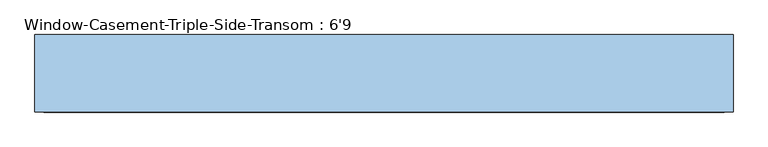
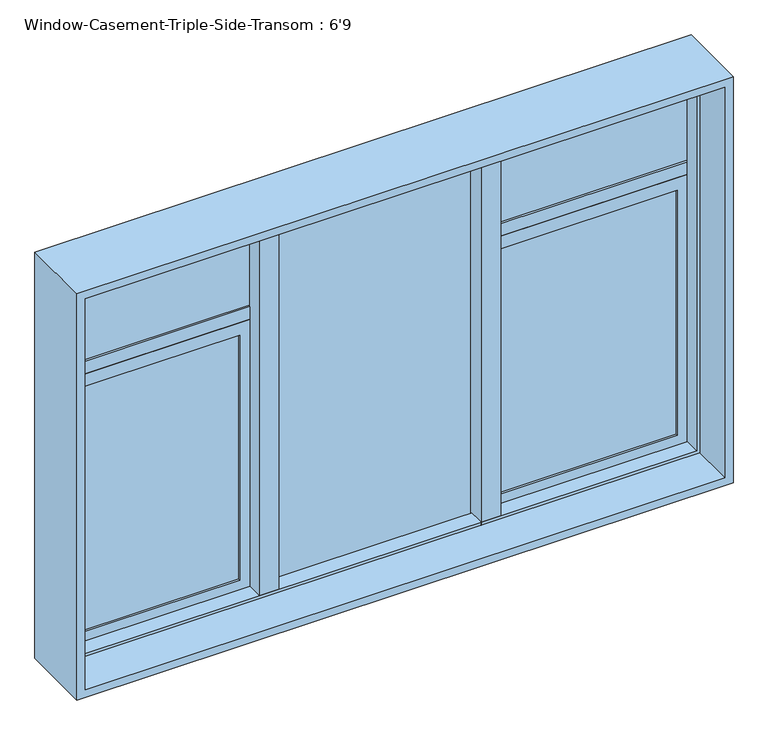
"""IFC4 building model written with IfcOpenShell, lengths in millimetres: window geometry, Window-Casement-Triple-Side-Transom : 6'9."""

from ifc_helpers import new_model, si_unit, frame, origin, place, context, project, spatial, polyline, outline, extrude, faceted_brep, source, transform, mapped, element, save


def window_casement_triple_side_transom_6_9_71562f8e(model_context):
    return source(origin(), model_context, "Body", "SolidModel", [
        faceted_brep([(-1003.3, 73.025, 2235.2), (-1003.3, 114.3, 2235.2), (1003.3, 114.3, 2235.2), (1003.3, 73.025, 2235.2), (-993.1796875, 22.225, 2225.0796875), (-993.1796875, 73.025, 2225.0796875), (993.1796875, 73.025, 2225.0796875), (993.1796875, 22.225, 2225.0796875), (-1003.3, -114.3, 2235.2), (-1003.3, 22.225, 2235.2), (1003.3, 22.225, 2235.2), (1003.3, -114.3, 2235.2), (-1028.7, 114.3, 2260.6), (-1028.7, -114.3, 2260.6), (1028.7, -114.3, 2260.6), (1028.7, 114.3, 2260.6), (1003.3, 114.3, 939.8), (1003.3, 73.025, 939.8), (993.1796875, 73.025, 949.9203125), (993.1796875, 22.225, 949.9203125), (1003.3, 22.225, 939.8), (1003.3, -114.3, 939.8), (1028.7, -114.3, 914.4), (1028.7, 114.3, 914.4), (-1003.3, 114.3, 939.8), (-1003.3, 73.025, 939.8), (-993.1796875, 73.025, 949.9203125), (-993.1796875, 22.225, 949.9203125), (-1003.3, 22.225, 939.8), (-1003.3, -114.3, 939.8), (-1028.7, -114.3, 914.4), (-1028.7, 114.3, 914.4)], [[[0, 1, 2, 3]], [[4, 5, 6, 7]], [[8, 9, 10, 11]], [[12, 13, 14, 15]], [[3, 2, 16, 17]], [[7, 6, 18, 19]], [[11, 10, 20, 21]], [[15, 14, 22, 23]], [[17, 16, 24, 25]], [[19, 18, 26, 27]], [[21, 20, 28, 29]], [[23, 22, 30, 31]], [[25, 24, 1, 0]], [[3, 17, 25, 0], [5, 26, 18, 6]], [[27, 26, 5, 4]], [[9, 28, 20, 10], [7, 19, 27, 4]], [[29, 28, 9, 8]], [[13, 30, 22, 14], [11, 21, 29, 8]], [[31, 30, 13, 12]], [[15, 23, 31, 12], [1, 24, 16, 2]]]),
        extrude(outline(polyline([(-317.5, 111.125), (-317.5, 22.225), (-378.4203125, 22.225), (-378.4203125, 73.025), (-368.3, 73.025), (-368.3, 111.125), (-317.5, 111.125)])), frame((0.0, 0.0, 939.8), z_axis=(0.0, 0.0, 1.0), x_axis=(1.0, 0.0, 0.0)), (0.0, 0.0, 1.0), 1295.4),
        extrude(outline(polyline([(368.3, 111.125), (368.3, 73.025), (378.4203125, 73.025), (378.4203125, 22.225), (317.5, 22.225), (317.5, 111.125), (368.3, 111.125)])), frame((0.0, 0.0, 939.8), z_axis=(0.0, 0.0, 1.0), x_axis=(1.0, 0.0, 0.0)), (0.0, 0.0, 1.0), 1295.4),
        extrude(outline(polyline([(1835.8048438, 368.3), (939.8, 368.3), (939.8, 1003.3), (1835.8048438, 1003.3), (1835.8048438, 368.3)]), holes=[polyline([(1793.9345313, 961.4296875), (981.6703125, 961.4296875), (981.6703125, 410.1703125), (1793.9345313, 410.1703125), (1793.9345313, 961.4296875)])]), frame((0.0, 73.025, 0.0), z_axis=(0.0, 1.0, 0.0), x_axis=(0.0, 0.0, 1.0)), (0.0, 0.0, 1.0), 31.75),
        extrude(outline(polyline([(1835.8048438, -1003.3), (939.8, -1003.3), (939.8, -368.3), (1835.8048438, -368.3), (1835.8048438, -1003.3)]), holes=[polyline([(1793.9345313, -410.1703125), (981.6703125, -410.1703125), (981.6703125, -961.4296875), (1793.9345313, -961.4296875), (1793.9345313, -410.1703125)])]), frame((0.0, 73.025, 0.0), z_axis=(0.0, 1.0, 0.0), x_axis=(0.0, 0.0, 1.0)), (0.0, 0.0, 1.0), 31.75),
        extrude(outline(polyline([(-410.1703125, 98.425), (-410.1703125, 92.075), (-961.4296875, 92.075), (-961.4296875, 98.425), (-410.1703125, 98.425)])), frame((0.0, 0.0, 981.6703125), z_axis=(0.0, 0.0, 1.0), x_axis=(1.0, 0.0, 0.0)), (0.0, 0.0, 1.0), 812.2642188),
        extrude(outline(polyline([(-410.1703125, 85.725), (-410.1703125, 79.375), (-961.4296875, 79.375), (-961.4296875, 85.725), (-410.1703125, 85.725)])), frame((0.0, 0.0, 981.6703125), z_axis=(0.0, 0.0, 1.0), x_axis=(1.0, 0.0, 0.0)), (0.0, 0.0, 1.0), 812.2642188),
        extrude(outline(polyline([(961.4296875, 98.425), (961.4296875, 92.075), (410.1703125, 92.075), (410.1703125, 98.425), (961.4296875, 98.425)])), frame((0.0, 0.0, 981.6703125), z_axis=(0.0, 0.0, 1.0), x_axis=(1.0, 0.0, 0.0)), (0.0, 0.0, 1.0), 812.2642188),
        extrude(outline(polyline([(961.4296875, 85.725), (961.4296875, 79.375), (410.1703125, 79.375), (410.1703125, 85.725), (961.4296875, 85.725)])), frame((0.0, 0.0, 981.6703125), z_axis=(0.0, 0.0, 1.0), x_axis=(1.0, 0.0, 0.0)), (0.0, 0.0, 1.0), 812.2642188),
        extrude(outline(polyline([(1003.3, 104.775), (1003.3, 73.025), (368.3, 73.025), (368.3, 104.775), (1003.3, 104.775)])), frame((0.0, 0.0, 1835.8048438), z_axis=(0.0, 0.0, 1.0), x_axis=(1.0, 0.0, 0.0)), (0.0, 0.0, 1.0), 41.8703125),
        extrude(outline(polyline([(317.5, 98.425), (317.5, 92.075), (-317.5, 92.075), (-317.5, 98.425), (317.5, 98.425)])), frame((0.0, 0.0, 939.8), z_axis=(0.0, 0.0, 1.0), x_axis=(1.0, 0.0, 0.0)), (0.0, 0.0, 1.0), 1295.4),
        extrude(outline(polyline([(317.5, 85.725), (317.5, 79.375), (-317.5, 79.375), (-317.5, 85.725), (317.5, 85.725)])), frame((0.0, 0.0, 939.8), z_axis=(0.0, 0.0, 1.0), x_axis=(1.0, 0.0, 0.0)), (0.0, 0.0, 1.0), 1295.4),
        extrude(outline(polyline([(-368.3, 104.775), (-368.3, 73.025), (-1003.3, 73.025), (-1003.3, 104.775), (-368.3, 104.775)])), frame((0.0, 0.0, 1835.8048438), z_axis=(0.0, 0.0, 1.0), x_axis=(1.0, 0.0, 0.0)), (0.0, 0.0, 1.0), 41.8703125),
        extrude(outline(polyline([(-368.3, 98.425), (-368.3, 92.075), (-1003.3, 92.075), (-1003.3, 98.425), (-368.3, 98.425)])), frame((0.0, 0.0, 1877.6751562), z_axis=(0.0, 0.0, 1.0), x_axis=(1.0, 0.0, 0.0)), (0.0, 0.0, 1.0), 357.5248438),
        extrude(outline(polyline([(-368.3, 85.725), (-368.3, 79.375), (-1003.3, 79.375), (-1003.3, 85.725), (-368.3, 85.725)])), frame((0.0, 0.0, 1877.6751562), z_axis=(0.0, 0.0, 1.0), x_axis=(1.0, 0.0, 0.0)), (0.0, 0.0, 1.0), 357.5248438),
        extrude(outline(polyline([(1003.3, 98.425), (1003.3, 92.075), (368.3, 92.075), (368.3, 98.425), (1003.3, 98.425)])), frame((0.0, 0.0, 1877.6751562), z_axis=(0.0, 0.0, 1.0), x_axis=(1.0, 0.0, 0.0)), (0.0, 0.0, 1.0), 357.5248438),
        extrude(outline(polyline([(1003.3, 85.725), (1003.3, 79.375), (368.3, 79.375), (368.3, 85.725), (1003.3, 85.725)])), frame((0.0, 0.0, 1877.6751562), z_axis=(0.0, 0.0, 1.0), x_axis=(1.0, 0.0, 0.0)), (0.0, 0.0, 1.0), 357.5248438),
    ])


if __name__ == "__main__":
    model = new_model("IFC4")
    model_context = context("Model", 3, world=origin())
    ifc_project = project(units=[si_unit("LENGTHUNIT", "METRE", prefix="MILLI")], contexts=[model_context])
    site = spatial("IfcSite", under=ifc_project)
    building = spatial("IfcBuilding", under=site)
    placement = place(None, origin())
    window_casement_triple_side_transom_6_9_shape = window_casement_triple_side_transom_6_9_71562f8e(model_context)
    element("IfcWindow", 1, ObjectType="Window-Casement-Triple-Side-Transom : 6'9", at=placement, inside=building, context=model_context, shape_type="MappedRepresentation", body=[
        mapped(window_casement_triple_side_transom_6_9_shape, transform((0.0, 0.0, 0.0), x_axis=(1.0, 0.0, 0.0), y_axis=(0.0, 1.0, 0.0), z_axis=(0.0, 0.0, 1.0))),
    ])
    save(model, "model.ifc")

# Revit data of these elements
# Type "Window-Casement-Triple-Side-Transom : 6'9"
#   Type Mark = "25"
#   Fire Rating = "0.5h"
#   Assembly Code = "B2020100"
#   Analytic Construction = "Double glazing - domestic"
#   Window Width = 2' - 3"
#   Window Inset [instance default] = 0' - 0 5/8"
#   Wall Thickness [instance default] = 0' - 6"
#   Visual Light Transmittance = 0.81
#   Transom Height Ratio = 0.3
#   Thermal Resistance (R) = 1.8146 (h·ft²·°F)/BTU
#   Solar Heat Gain Coefficient = 0.76
#   Rough Width = 6' - 9 1/2"
#   Rough Height = 4' - 5 1/2"
#   Open Window Height = 3' - 1.1"
#   Heat Transfer Coefficient (U) = 0.5511 BTU/(h·ft²·°F)
#   Height = 4' - 5"
#   Transom Height = 1' - 3.9"
#   Frame Gap 3 [instance default] = 0' - 1 83/128"
#   Frame Gap 2 [instance default] = 0' - 0 5/8"
#   Frame Gap 1 = 0' - 1 51/128"
#   Default Sill Height = 3' - 0"
#   Width = 6' - 9"
#   Frame Material = Metal - Aluminum
#   Glass Panel Material = Glass
#   Wall Closure = (empty or 0)
# Element 1 (IfcWindow, "Window-Casement-Triple-Side-Transom : 6'9")
#   Wall Thickness = 0' - 9"
#   Materials on its faces: "Metal - Aluminum", "Glass"
# Materials
#   "Metal - Aluminum": class "Metal", colour RGB 247 247 247, transparency 0
#   "Glass": class "Glass", colour RGB 154 182 205, transparency 0.85, Description = "Soda Lime Glass", Cost = 0
